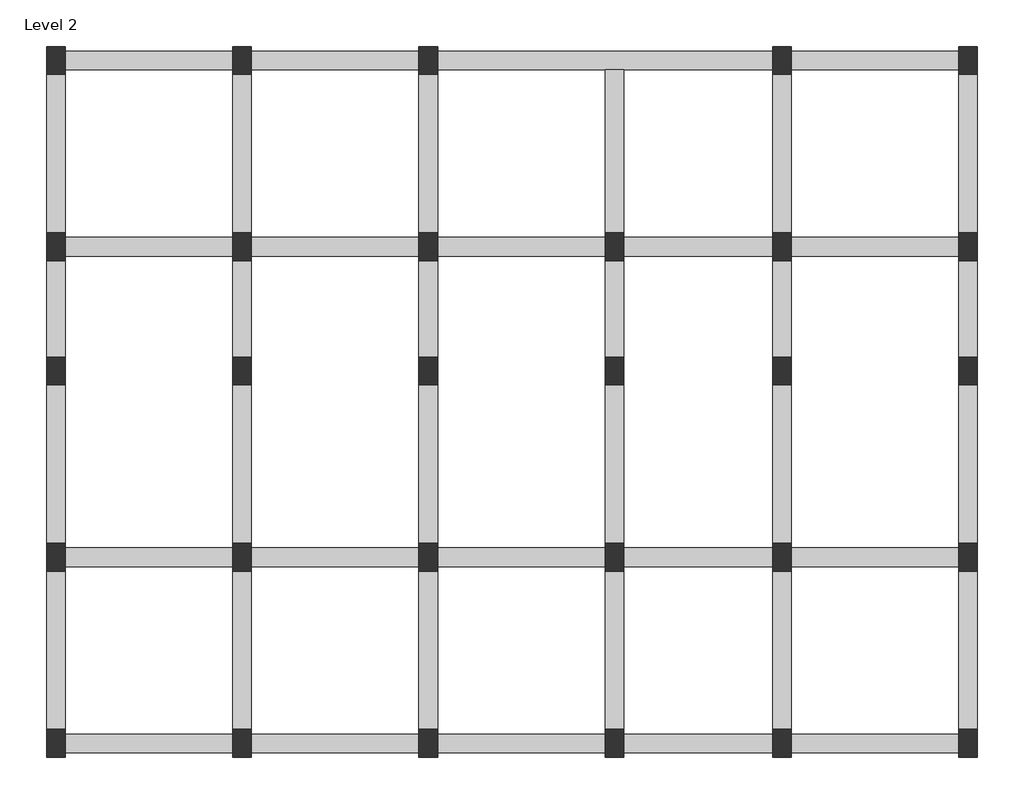
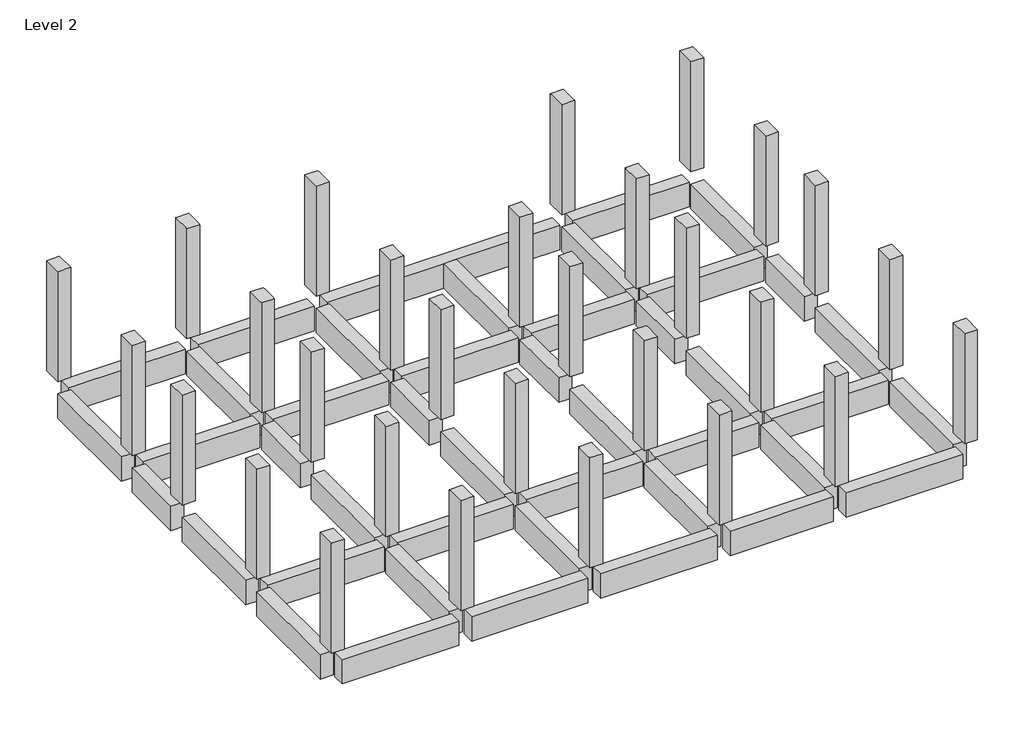
# One storey: 29 columns, 10 beams.
"""IFC4 building model written with IfcOpenShell, lengths in millimetres."""

from ifc_helpers import new_model, si_unit, frame, origin, place, context, project, spatial, polyline, outline, extrude, faceted_brep, element, save

model = new_model("IFC4")

# Units and contexts
model_context = context("Model", 3, world=origin())
ifc_project = project(units=[si_unit("LENGTHUNIT", "METRE", prefix="MILLI")], contexts=[model_context])

# Site, building, storey
site = spatial("IfcSite", under=ifc_project)
building = spatial("IfcBuilding", under=site)
storey = spatial("IfcBuildingStorey", under=building, Name="Level 2", Elevation=3048.0)

# Beams
placement = place(None, origin())
element("IfcBeam", 1, ObjectType="Concrete-Rectangular Beam : 12 x 24", at=placement, inside=storey, context=model_context, shape_type="SweptSolid", body=[
    extrude(outline(polyline([(2607.7603583, 7596.6647757), (2607.7603583, 7291.8647757), (-135.4396417, 7291.8647757), (-135.4396417, 7596.6647757), (2607.7603583, 7596.6647757)])), frame((0.0, 0.0, 2133.6), z_axis=(0.0, 0.0, 1.0), x_axis=(1.0, 0.0, 0.0)), (0.0, 0.0, 1.0), 609.6),
    extrude(outline(polyline([(-12022.6396417, 7291.8647757), (-12022.6396417, 7596.6647757), (-9279.4396417, 7596.6647757), (-9279.4396417, 7291.8647757), (-12022.6396417, 7291.8647757)])), frame((0.0, 0.0, 2133.6), z_axis=(0.0, 0.0, 1.0), x_axis=(1.0, 0.0, 0.0)), (0.0, 0.0, 1.0), 609.6),
    extrude(outline(polyline([(-8974.6396417, 7291.8647757), (-8974.6396417, 7596.6647757), (-6231.4396417, 7596.6647757), (-6231.4396417, 7291.8647757), (-8974.6396417, 7291.8647757)])), frame((0.0, 0.0, 2133.6), z_axis=(0.0, 0.0, 1.0), x_axis=(1.0, 0.0, 0.0)), (0.0, 0.0, 1.0), 609.6),
    extrude(outline(polyline([(-5926.6396417, 7291.8647757), (-5926.6396417, 7596.6647757), (-3183.4396417, 7596.6647757), (-3183.4396417, 7291.8647757), (-5926.6396417, 7291.8647757)])), frame((0.0, 0.0, 2133.6), z_axis=(0.0, 0.0, 1.0), x_axis=(1.0, 0.0, 0.0)), (0.0, 0.0, 1.0), 609.6),
    extrude(outline(polyline([(-2878.6396417, 7291.8647757), (-2878.6396417, 7596.6647757), (-440.2396417, 7596.6647757), (-440.2396417, 7291.8647757), (-2878.6396417, 7291.8647757)])), frame((0.0, 0.0, 2133.6), z_axis=(0.0, 0.0, 1.0), x_axis=(1.0, 0.0, 0.0)), (0.0, 0.0, 1.0), 609.6),
])
element("IfcBeam", 2, ObjectType="Concrete-Rectangular Beam : 12 x 24", at=placement, inside=storey, context=model_context, shape_type="SweptSolid", body=[
    extrude(outline(polyline([(2607.7603583, 10644.6647757), (2607.7603583, 10339.8647757), (-135.4396417, 10339.8647757), (-135.4396417, 10644.6647757), (2607.7603583, 10644.6647757)])), frame((0.0, 0.0, 2133.6), z_axis=(0.0, 0.0, 1.0), x_axis=(1.0, 0.0, 0.0)), (0.0, 0.0, 1.0), 609.6),
    extrude(outline(polyline([(-12022.6396417, 10339.8647757), (-12022.6396417, 10644.6647757), (-9279.4396417, 10644.6647757), (-9279.4396417, 10339.8647757), (-12022.6396417, 10339.8647757)])), frame((0.0, 0.0, 2133.6), z_axis=(0.0, 0.0, 1.0), x_axis=(1.0, 0.0, 0.0)), (0.0, 0.0, 1.0), 609.6),
    extrude(outline(polyline([(-8974.6396417, 10339.8647757), (-8974.6396417, 10644.6647757), (-6231.4396417, 10644.6647757), (-6231.4396417, 10339.8647757), (-8974.6396417, 10339.8647757)])), frame((0.0, 0.0, 2133.6), z_axis=(0.0, 0.0, 1.0), x_axis=(1.0, 0.0, 0.0)), (0.0, 0.0, 1.0), 609.6),
    extrude(outline(polyline([(-5926.6396417, 10339.8647757), (-5926.6396417, 10644.6647757), (-3183.4396417, 10644.6647757), (-3183.4396417, 10339.8647757), (-5926.6396417, 10339.8647757)])), frame((0.0, 0.0, 2133.6), z_axis=(0.0, 0.0, 1.0), x_axis=(1.0, 0.0, 0.0)), (0.0, 0.0, 1.0), 609.6),
    extrude(outline(polyline([(-2878.6396417, 10339.8647757), (-2878.6396417, 10644.6647757), (-440.2396417, 10644.6647757), (-440.2396417, 10339.8647757), (-2878.6396417, 10339.8647757)])), frame((0.0, 0.0, 2133.6), z_axis=(0.0, 0.0, 1.0), x_axis=(1.0, 0.0, 0.0)), (0.0, 0.0, 1.0), 609.6),
])
element("IfcBeam", 3, ObjectType="Concrete-Rectangular Beam : 12 x 24", at=placement, inside=storey, context=model_context, shape_type="SweptSolid", body=[
    extrude(outline(polyline([(2607.7603583, 15727.9119241), (2607.7603583, 15423.1119241), (-135.4396417, 15423.1119241), (-135.4396417, 15727.9119241), (2607.7603583, 15727.9119241)])), frame((0.0, 0.0, 2133.6), z_axis=(0.0, 0.0, 1.0), x_axis=(1.0, 0.0, 0.0)), (0.0, 0.0, 1.0), 609.6),
    extrude(outline(polyline([(-12022.6396417, 15423.1119241), (-12022.6396417, 15727.9119241), (-9279.4396417, 15727.9119241), (-9279.4396417, 15423.1119241), (-12022.6396417, 15423.1119241)])), frame((0.0, 0.0, 2133.6), z_axis=(0.0, 0.0, 1.0), x_axis=(1.0, 0.0, 0.0)), (0.0, 0.0, 1.0), 609.6),
    extrude(outline(polyline([(-8974.6396417, 15423.1119241), (-8974.6396417, 15727.9119241), (-6231.4396417, 15727.9119241), (-6231.4396417, 15423.1119241), (-8974.6396417, 15423.1119241)])), frame((0.0, 0.0, 2133.6), z_axis=(0.0, 0.0, 1.0), x_axis=(1.0, 0.0, 0.0)), (0.0, 0.0, 1.0), 609.6),
    extrude(outline(polyline([(-5926.6396417, 15423.1119241), (-5926.6396417, 15727.9119241), (-3183.4396417, 15727.9119241), (-3183.4396417, 15423.1119241), (-5926.6396417, 15423.1119241)])), frame((0.0, 0.0, 2133.6), z_axis=(0.0, 0.0, 1.0), x_axis=(1.0, 0.0, 0.0)), (0.0, 0.0, 1.0), 609.6),
    extrude(outline(polyline([(-2878.6396417, 15423.1119241), (-2878.6396417, 15727.9119241), (-440.2396417, 15727.9119241), (-440.2396417, 15423.1119241), (-2878.6396417, 15423.1119241)])), frame((0.0, 0.0, 2133.6), z_axis=(0.0, 0.0, 1.0), x_axis=(1.0, 0.0, 0.0)), (0.0, 0.0, 1.0), 609.6),
])
element("IfcBeam", 4, ObjectType="Concrete-Rectangular Beam : 12 x 24", at=placement, inside=storey, context=model_context, shape_type="Brep", body=[
    faceted_brep([(2607.7603583, 18471.1119241, 2743.2), (2607.7603583, 18775.9119241, 2743.2), (-135.4396417, 18775.9119241, 2743.2), (-135.4396417, 18471.1119241, 2743.2), (2607.7603583, 18471.1119241, 2133.6), (-135.4396417, 18471.1119241, 2133.6), (2607.7603583, 18775.9119241, 2133.6), (-135.4396417, 18775.9119241, 2133.6)], [[[0, 1, 2, 3]], [[4, 0, 3, 5]], [[6, 4, 5, 7]], [[1, 6, 7, 2]], [[1, 0, 4, 6]], [[3, 2, 7, 5]]]),
    faceted_brep([(-12022.6396417, 18471.1119241, 2743.2), (-12022.6396417, 18775.9119241, 2743.2), (-12022.6396417, 18775.9119241, 2133.6), (-12022.6396417, 18471.1119241, 2133.6), (-9279.4396417, 18775.9119241, 2743.2), (-9279.4396417, 18471.1119241, 2743.2), (-9279.4396417, 18471.1119241, 2133.6), (-9279.4396417, 18775.9119241, 2133.6)], [[[0, 1, 2, 3]], [[4, 5, 6, 7]], [[1, 0, 5, 4]], [[0, 3, 6, 5]], [[3, 2, 7, 6]], [[2, 1, 4, 7]]]),
    faceted_brep([(-8974.6396417, 18471.1119241, 2743.2), (-8974.6396417, 18775.9119241, 2743.2), (-8974.6396417, 18775.9119241, 2133.6), (-8974.6396417, 18471.1119241, 2133.6), (-6231.4396417, 18775.9119241, 2743.2), (-6231.4396417, 18471.1119241, 2743.2), (-6231.4396417, 18471.1119241, 2133.6), (-6231.4396417, 18775.9119241, 2133.6)], [[[0, 1, 2, 3]], [[4, 5, 6, 7]], [[1, 0, 5, 4]], [[0, 3, 6, 5]], [[3, 2, 7, 6]], [[2, 1, 4, 7]]]),
    faceted_brep([(-5926.6396417, 18471.1119241, 2743.2), (-5926.6396417, 18775.9119241, 2743.2), (-5926.6396417, 18775.9119241, 2133.6), (-5926.6396417, 18471.1119241, 2133.6), (-440.2396417, 18775.9119241, 2743.2), (-440.2396417, 18471.1119241, 2743.2), (-440.2396417, 18471.1119241, 2133.6), (-440.2396417, 18775.9119241, 2133.6), (-3183.4396417, 18471.1119241, 2743.2), (-2878.6396417, 18471.1119241, 2743.2), (-3183.4396417, 18471.1119241, 2133.6), (-2878.6396417, 18471.1119241, 2133.6)], [[[0, 1, 2, 3]], [[4, 5, 6, 7]], [[1, 0, 8, 9, 5, 4]], [[0, 3, 10, 11, 6, 5, 9, 8]], [[3, 2, 7, 6, 11, 10]], [[2, 1, 4, 7]]]),
])
element("IfcBeam", 5, ObjectType="Concrete-Rectangular Beam : 12 x 24", at=placement, inside=storey, context=model_context, shape_type="SweptSolid", body=[
    extrude(outline(polyline([(-12022.6396417, 7672.8647757), (-12327.4396417, 7672.8647757), (-12327.4396417, 10263.6647757), (-12022.6396417, 10263.6647757), (-12022.6396417, 7672.8647757)])), frame((0.0, 0.0, 2133.6), z_axis=(0.0, 0.0, 1.0), x_axis=(1.0, 0.0, 0.0)), (0.0, 0.0, 1.0), 609.6),
    extrude(outline(polyline([(-12327.4396417, 18394.9119241), (-12022.6396417, 18394.9119241), (-12022.6396417, 15804.1119241), (-12327.4396417, 15804.1119241), (-12327.4396417, 18394.9119241)])), frame((0.0, 0.0, 2133.6), z_axis=(0.0, 0.0, 1.0), x_axis=(1.0, 0.0, 0.0)), (0.0, 0.0, 1.0), 609.6),
    extrude(outline(polyline([(-12022.6396417, 10720.8647757), (-12327.4396417, 10720.8647757), (-12327.4396417, 13311.6647757), (-12022.6396417, 13311.6647757), (-12022.6396417, 10720.8647757)])), frame((0.0, 0.0, 2133.6), z_axis=(0.0, 0.0, 1.0), x_axis=(1.0, 0.0, 0.0)), (0.0, 0.0, 1.0), 609.6),
    extrude(outline(polyline([(-12022.6396417, 13768.8647757), (-12327.4396417, 13768.8647757), (-12327.4396417, 15346.9119241), (-12022.6396417, 15346.9119241), (-12022.6396417, 13768.8647757)])), frame((0.0, 0.0, 2133.6), z_axis=(0.0, 0.0, 1.0), x_axis=(1.0, 0.0, 0.0)), (0.0, 0.0, 1.0), 609.6),
])
element("IfcBeam", 6, ObjectType="Concrete-Rectangular Beam : 12 x 24", at=placement, inside=storey, context=model_context, shape_type="SweptSolid", body=[
    extrude(outline(polyline([(-8974.6396417, 7672.8647757), (-9279.4396417, 7672.8647757), (-9279.4396417, 10263.6647757), (-8974.6396417, 10263.6647757), (-8974.6396417, 7672.8647757)])), frame((0.0, 0.0, 2133.6), z_axis=(0.0, 0.0, 1.0), x_axis=(1.0, 0.0, 0.0)), (0.0, 0.0, 1.0), 609.6),
    extrude(outline(polyline([(-9279.4396417, 18394.9119241), (-8974.6396417, 18394.9119241), (-8974.6396417, 15804.1119241), (-9279.4396417, 15804.1119241), (-9279.4396417, 18394.9119241)])), frame((0.0, 0.0, 2133.6), z_axis=(0.0, 0.0, 1.0), x_axis=(1.0, 0.0, 0.0)), (0.0, 0.0, 1.0), 609.6),
    extrude(outline(polyline([(-8974.6396417, 10720.8647757), (-9279.4396417, 10720.8647757), (-9279.4396417, 13311.6647757), (-8974.6396417, 13311.6647757), (-8974.6396417, 10720.8647757)])), frame((0.0, 0.0, 2133.6), z_axis=(0.0, 0.0, 1.0), x_axis=(1.0, 0.0, 0.0)), (0.0, 0.0, 1.0), 609.6),
    extrude(outline(polyline([(-8974.6396417, 13768.8647757), (-9279.4396417, 13768.8647757), (-9279.4396417, 15346.9119241), (-8974.6396417, 15346.9119241), (-8974.6396417, 13768.8647757)])), frame((0.0, 0.0, 2133.6), z_axis=(0.0, 0.0, 1.0), x_axis=(1.0, 0.0, 0.0)), (0.0, 0.0, 1.0), 609.6),
])
element("IfcBeam", 7, ObjectType="Concrete-Rectangular Beam : 12 x 24", at=placement, inside=storey, context=model_context, shape_type="SweptSolid", body=[
    extrude(outline(polyline([(-5926.6396417, 7672.8647757), (-6231.4396417, 7672.8647757), (-6231.4396417, 10263.6647757), (-5926.6396417, 10263.6647757), (-5926.6396417, 7672.8647757)])), frame((0.0, 0.0, 2133.6), z_axis=(0.0, 0.0, 1.0), x_axis=(1.0, 0.0, 0.0)), (0.0, 0.0, 1.0), 609.6),
    extrude(outline(polyline([(-6231.4396417, 18394.9119241), (-5926.6396417, 18394.9119241), (-5926.6396417, 15804.1119241), (-6231.4396417, 15804.1119241), (-6231.4396417, 18394.9119241)])), frame((0.0, 0.0, 2133.6), z_axis=(0.0, 0.0, 1.0), x_axis=(1.0, 0.0, 0.0)), (0.0, 0.0, 1.0), 609.6),
    extrude(outline(polyline([(-5926.6396417, 10720.8647757), (-6231.4396417, 10720.8647757), (-6231.4396417, 13311.6647757), (-5926.6396417, 13311.6647757), (-5926.6396417, 10720.8647757)])), frame((0.0, 0.0, 2133.6), z_axis=(0.0, 0.0, 1.0), x_axis=(1.0, 0.0, 0.0)), (0.0, 0.0, 1.0), 609.6),
    extrude(outline(polyline([(-5926.6396417, 13768.8647757), (-6231.4396417, 13768.8647757), (-6231.4396417, 15346.9119241), (-5926.6396417, 15346.9119241), (-5926.6396417, 13768.8647757)])), frame((0.0, 0.0, 2133.6), z_axis=(0.0, 0.0, 1.0), x_axis=(1.0, 0.0, 0.0)), (0.0, 0.0, 1.0), 609.6),
])
element("IfcBeam", 8, ObjectType="Concrete-Rectangular Beam : 12 x 24", at=placement, inside=storey, context=model_context, shape_type="SweptSolid", body=[
    extrude(outline(polyline([(-2878.6396417, 7672.8647757), (-3183.4396417, 7672.8647757), (-3183.4396417, 10263.6647757), (-2878.6396417, 10263.6647757), (-2878.6396417, 7672.8647757)])), frame((0.0, 0.0, 2133.6), z_axis=(0.0, 0.0, 1.0), x_axis=(1.0, 0.0, 0.0)), (0.0, 0.0, 1.0), 609.6),
    extrude(outline(polyline([(-2878.6396417, 10720.8647757), (-3183.4396417, 10720.8647757), (-3183.4396417, 13311.6647757), (-2878.6396417, 13311.6647757), (-2878.6396417, 10720.8647757)])), frame((0.0, 0.0, 2133.6), z_axis=(0.0, 0.0, 1.0), x_axis=(1.0, 0.0, 0.0)), (0.0, 0.0, 1.0), 609.6),
    extrude(outline(polyline([(-2878.6396417, 13768.8647757), (-3183.4396417, 13768.8647757), (-3183.4396417, 15346.9119241), (-2878.6396417, 15346.9119241), (-2878.6396417, 13768.8647757)])), frame((0.0, 0.0, 2133.6), z_axis=(0.0, 0.0, 1.0), x_axis=(1.0, 0.0, 0.0)), (0.0, 0.0, 1.0), 609.6),
    extrude(outline(polyline([(-2878.6396417, 15804.1119241), (-3183.4396417, 15804.1119241), (-3183.4396417, 18471.1119241), (-2878.6396417, 18471.1119241), (-2878.6396417, 15804.1119241)])), frame((0.0, 0.0, 2133.6), z_axis=(0.0, 0.0, 1.0), x_axis=(1.0, 0.0, 0.0)), (0.0, 0.0, 1.0), 609.6),
])
element("IfcBeam", 9, ObjectType="Concrete-Rectangular Beam : 12 x 24", at=placement, inside=storey, context=model_context, shape_type="SweptSolid", body=[
    extrude(outline(polyline([(-135.4396417, 7672.8647757), (-440.2396417, 7672.8647757), (-440.2396417, 10263.6647757), (-135.4396417, 10263.6647757), (-135.4396417, 7672.8647757)])), frame((0.0, 0.0, 2133.6), z_axis=(0.0, 0.0, 1.0), x_axis=(1.0, 0.0, 0.0)), (0.0, 0.0, 1.0), 609.6),
    extrude(outline(polyline([(-440.2396417, 18394.9119241), (-135.4396417, 18394.9119241), (-135.4396417, 15804.1119241), (-440.2396417, 15804.1119241), (-440.2396417, 18394.9119241)])), frame((0.0, 0.0, 2133.6), z_axis=(0.0, 0.0, 1.0), x_axis=(1.0, 0.0, 0.0)), (0.0, 0.0, 1.0), 609.6),
    extrude(outline(polyline([(-135.4396417, 10720.8647757), (-440.2396417, 10720.8647757), (-440.2396417, 13311.6647757), (-135.4396417, 13311.6647757), (-135.4396417, 10720.8647757)])), frame((0.0, 0.0, 2133.6), z_axis=(0.0, 0.0, 1.0), x_axis=(1.0, 0.0, 0.0)), (0.0, 0.0, 1.0), 609.6),
    extrude(outline(polyline([(-135.4396417, 13768.8647757), (-440.2396417, 13768.8647757), (-440.2396417, 15346.9119241), (-135.4396417, 15346.9119241), (-135.4396417, 13768.8647757)])), frame((0.0, 0.0, 2133.6), z_axis=(0.0, 0.0, 1.0), x_axis=(1.0, 0.0, 0.0)), (0.0, 0.0, 1.0), 609.6),
])
element("IfcBeam", 10, ObjectType="Concrete-Rectangular Beam : 12 x 24", at=placement, inside=storey, context=model_context, shape_type="SweptSolid", body=[
    extrude(outline(polyline([(2912.5603583, 7672.8647757), (2607.7603583, 7672.8647757), (2607.7603583, 10263.6647757), (2912.5603583, 10263.6647757), (2912.5603583, 7672.8647757)])), frame((0.0, 0.0, 2133.6), z_axis=(0.0, 0.0, 1.0), x_axis=(1.0, 0.0, 0.0)), (0.0, 0.0, 1.0), 609.6),
    extrude(outline(polyline([(2607.7603583, 18394.9119241), (2912.5603583, 18394.9119241), (2912.5603583, 15804.1119241), (2607.7603583, 15804.1119241), (2607.7603583, 18394.9119241)])), frame((0.0, 0.0, 2133.6), z_axis=(0.0, 0.0, 1.0), x_axis=(1.0, 0.0, 0.0)), (0.0, 0.0, 1.0), 609.6),
    extrude(outline(polyline([(2912.5603583, 10720.8647757), (2607.7603583, 10720.8647757), (2607.7603583, 13311.6647757), (2912.5603583, 13311.6647757), (2912.5603583, 10720.8647757)])), frame((0.0, 0.0, 2133.6), z_axis=(0.0, 0.0, 1.0), x_axis=(1.0, 0.0, 0.0)), (0.0, 0.0, 1.0), 609.6),
    extrude(outline(polyline([(2912.5603583, 13768.8647757), (2607.7603583, 13768.8647757), (2607.7603583, 15346.9119241), (2912.5603583, 15346.9119241), (2912.5603583, 13768.8647757)])), frame((0.0, 0.0, 2133.6), z_axis=(0.0, 0.0, 1.0), x_axis=(1.0, 0.0, 0.0)), (0.0, 0.0, 1.0), 609.6),
])

# Columns
element("IfcColumn", 11, ObjectType="Concrete-Rectangular-Column : c1", at=placement, inside=storey, context=model_context, shape_type="SweptSolid", body=[
    extrude(outline(polyline([(-12327.4396417, 7215.6647757), (-12327.4396417, 7672.8647757), (-12022.6396417, 7672.8647757), (-12022.6396417, 7215.6647757), (-12327.4396417, 7215.6647757)])), frame((0.0, 0.0, 3048.0), z_axis=(0.0, 0.0, 1.0), x_axis=(1.0, 0.0, 0.0)), (0.0, 0.0, 1.0), 2743.2),
])
element("IfcColumn", 12, ObjectType="Concrete-Rectangular-Column : c1", at=placement, inside=storey, context=model_context, shape_type="Brep", body=[
    faceted_brep([(-9279.4396417, 7215.6647757, 3048.0), (-9279.4396417, 7672.8647757, 3048.0), (-8974.6396417, 7672.8647757, 3048.0), (-8974.6396417, 7215.6647757, 3048.0), (-9279.4396417, 7215.6647757, 5791.2), (-9279.4396417, 7291.8647757, 5791.2), (-9279.4396417, 7596.6647757, 5791.2), (-9279.4396417, 7672.8647757, 5791.2), (-8974.6396417, 7672.8647757, 5791.2), (-8974.6396417, 7596.6647757, 5791.2), (-8974.6396417, 7291.8647757, 5791.2), (-8974.6396417, 7215.6647757, 5791.2)], [[[0, 1, 2, 3]], [[4, 5, 6, 7, 1, 0]], [[7, 8, 2, 1]], [[8, 9, 10, 11, 3, 2]], [[11, 4, 0, 3]], [[4, 11, 10, 9, 8, 7, 6, 5]]]),
])
element("IfcColumn", 13, ObjectType="Concrete-Rectangular-Column : c1", at=placement, inside=storey, context=model_context, shape_type="Brep", body=[
    faceted_brep([(-6231.4396417, 7215.6647757, 3048.0), (-6231.4396417, 7672.8647757, 3048.0), (-5926.6396417, 7672.8647757, 3048.0), (-5926.6396417, 7215.6647757, 3048.0), (-6231.4396417, 7215.6647757, 5791.2), (-6231.4396417, 7291.8647757, 5791.2), (-6231.4396417, 7596.6647757, 5791.2), (-6231.4396417, 7672.8647757, 5791.2), (-5926.6396417, 7672.8647757, 5791.2), (-5926.6396417, 7596.6647757, 5791.2), (-5926.6396417, 7291.8647757, 5791.2), (-5926.6396417, 7215.6647757, 5791.2)], [[[0, 1, 2, 3]], [[4, 5, 6, 7, 1, 0]], [[7, 8, 2, 1]], [[8, 9, 10, 11, 3, 2]], [[11, 4, 0, 3]], [[4, 11, 10, 9, 8, 7, 6, 5]]]),
])
element("IfcColumn", 14, ObjectType="Concrete-Rectangular-Column : c1", at=placement, inside=storey, context=model_context, shape_type="Brep", body=[
    faceted_brep([(-3183.4396417, 7215.6647757, 3048.0), (-3183.4396417, 7672.8647757, 3048.0), (-2878.6396417, 7672.8647757, 3048.0), (-2878.6396417, 7215.6647757, 3048.0), (-3183.4396417, 7215.6647757, 5791.2), (-3183.4396417, 7291.8647757, 5791.2), (-3183.4396417, 7596.6647757, 5791.2), (-3183.4396417, 7672.8647757, 5791.2), (-2878.6396417, 7672.8647757, 5791.2), (-2878.6396417, 7596.6647757, 5791.2), (-2878.6396417, 7291.8647757, 5791.2), (-2878.6396417, 7215.6647757, 5791.2)], [[[0, 1, 2, 3]], [[4, 5, 6, 7, 1, 0]], [[7, 8, 2, 1]], [[8, 9, 10, 11, 3, 2]], [[11, 4, 0, 3]], [[4, 11, 10, 9, 8, 7, 6, 5]]]),
])
element("IfcColumn", 15, ObjectType="Concrete-Rectangular-Column : c1", at=placement, inside=storey, context=model_context, shape_type="Brep", body=[
    faceted_brep([(-440.2396417, 7215.6647757, 3048.0), (-440.2396417, 7672.8647757, 3048.0), (-135.4396417, 7672.8647757, 3048.0), (-135.4396417, 7215.6647757, 3048.0), (-440.2396417, 7215.6647757, 5791.2), (-440.2396417, 7291.8647757, 5791.2), (-440.2396417, 7596.6647757, 5791.2), (-440.2396417, 7672.8647757, 5791.2), (-135.4396417, 7672.8647757, 5791.2), (-135.4396417, 7596.6647757, 5791.2), (-135.4396417, 7291.8647757, 5791.2), (-135.4396417, 7215.6647757, 5791.2)], [[[0, 1, 2, 3]], [[4, 5, 6, 7, 1, 0]], [[7, 8, 2, 1]], [[8, 9, 10, 11, 3, 2]], [[11, 4, 0, 3]], [[4, 11, 10, 9, 8, 7, 6, 5]]]),
])
element("IfcColumn", 16, ObjectType="Concrete-Rectangular-Column : c1", at=placement, inside=storey, context=model_context, shape_type="SweptSolid", body=[
    extrude(outline(polyline([(2607.7603583, 7215.6647757), (2607.7603583, 7672.8647757), (2912.5603583, 7672.8647757), (2912.5603583, 7215.6647757), (2607.7603583, 7215.6647757)])), frame((0.0, 0.0, 3048.0), z_axis=(0.0, 0.0, 1.0), x_axis=(1.0, 0.0, 0.0)), (0.0, 0.0, 1.0), 2743.2),
])
element("IfcColumn", 17, ObjectType="Concrete-Rectangular-Column : c1", at=placement, inside=storey, context=model_context, shape_type="Brep", body=[
    faceted_brep([(-12327.4396417, 10263.6647757, 3048.0), (-12327.4396417, 10720.8647757, 3048.0), (-12022.6396417, 10720.8647757, 3048.0), (-12022.6396417, 10263.6647757, 3048.0), (-12327.4396417, 10263.6647757, 5791.2), (-12327.4396417, 10720.8647757, 5791.2), (-12327.4396417, 10720.8647757, 5181.6), (-12327.4396417, 10263.6647757, 5181.6), (-12022.6396417, 10720.8647757, 5791.2), (-12022.6396417, 10720.8647757, 5181.6), (-12022.6396417, 10263.6647757, 5791.2), (-12022.6396417, 10263.6647757, 5181.6)], [[[0, 1, 2, 3]], [[4, 5, 6, 1, 0, 7]], [[5, 8, 9, 2, 1, 6]], [[8, 10, 11, 3, 2, 9]], [[10, 4, 7, 0, 3, 11]], [[4, 10, 8, 5]]]),
])
element("IfcColumn", 18, ObjectType="Concrete-Rectangular-Column : c1", at=placement, inside=storey, context=model_context, shape_type="Brep", body=[
    faceted_brep([(-9279.4396417, 10263.6647757, 3048.0), (-9279.4396417, 10720.8647757, 3048.0), (-8974.6396417, 10720.8647757, 3048.0), (-8974.6396417, 10263.6647757, 3048.0), (-9279.4396417, 10263.6647757, 5791.2), (-9279.4396417, 10339.8647757, 5791.2), (-9279.4396417, 10644.6647757, 5791.2), (-9279.4396417, 10720.8647757, 5791.2), (-9279.4396417, 10720.8647757, 5181.6), (-9279.4396417, 10263.6647757, 5181.6), (-8974.6396417, 10720.8647757, 5791.2), (-8974.6396417, 10720.8647757, 5181.6), (-8974.6396417, 10644.6647757, 5791.2), (-8974.6396417, 10339.8647757, 5791.2), (-8974.6396417, 10263.6647757, 5791.2), (-8974.6396417, 10263.6647757, 5181.6)], [[[0, 1, 2, 3]], [[4, 5, 6, 7, 8, 1, 0, 9]], [[7, 10, 11, 2, 1, 8]], [[10, 12, 13, 14, 15, 3, 2, 11]], [[14, 4, 9, 0, 3, 15]], [[4, 14, 13, 12, 10, 7, 6, 5]]]),
])
element("IfcColumn", 19, ObjectType="Concrete-Rectangular-Column : c1", at=placement, inside=storey, context=model_context, shape_type="Brep", body=[
    faceted_brep([(-6231.4396417, 10263.6647757, 3048.0), (-6231.4396417, 10720.8647757, 3048.0), (-5926.6396417, 10720.8647757, 3048.0), (-5926.6396417, 10263.6647757, 3048.0), (-6231.4396417, 10263.6647757, 5791.2), (-6231.4396417, 10339.8647757, 5791.2), (-6231.4396417, 10644.6647757, 5791.2), (-6231.4396417, 10720.8647757, 5791.2), (-6231.4396417, 10720.8647757, 5181.6), (-6231.4396417, 10263.6647757, 5181.6), (-5926.6396417, 10720.8647757, 5791.2), (-5926.6396417, 10720.8647757, 5181.6), (-5926.6396417, 10644.6647757, 5791.2), (-5926.6396417, 10339.8647757, 5791.2), (-5926.6396417, 10263.6647757, 5791.2), (-5926.6396417, 10263.6647757, 5181.6)], [[[0, 1, 2, 3]], [[4, 5, 6, 7, 8, 1, 0, 9]], [[7, 10, 11, 2, 1, 8]], [[10, 12, 13, 14, 15, 3, 2, 11]], [[14, 4, 9, 0, 3, 15]], [[4, 14, 13, 12, 10, 7, 6, 5]]]),
])
element("IfcColumn", 20, ObjectType="Concrete-Rectangular-Column : c1", at=placement, inside=storey, context=model_context, shape_type="Brep", body=[
    faceted_brep([(-3183.4396417, 10263.6647757, 3048.0), (-3183.4396417, 10720.8647757, 3048.0), (-2878.6396417, 10720.8647757, 3048.0), (-2878.6396417, 10263.6647757, 3048.0), (-3183.4396417, 10263.6647757, 5791.2), (-3183.4396417, 10339.8647757, 5791.2), (-3183.4396417, 10644.6647757, 5791.2), (-3183.4396417, 10720.8647757, 5791.2), (-2878.6396417, 10720.8647757, 5791.2), (-2878.6396417, 10644.6647757, 5791.2), (-2878.6396417, 10339.8647757, 5791.2), (-2878.6396417, 10263.6647757, 5791.2)], [[[0, 1, 2, 3]], [[4, 5, 6, 7, 1, 0]], [[7, 8, 2, 1]], [[8, 9, 10, 11, 3, 2]], [[11, 4, 0, 3]], [[4, 11, 10, 9, 8, 7, 6, 5]]]),
])
element("IfcColumn", 21, ObjectType="Concrete-Rectangular-Column : c1", at=placement, inside=storey, context=model_context, shape_type="Brep", body=[
    faceted_brep([(-440.2396417, 10263.6647757, 3048.0), (-440.2396417, 10720.8647757, 3048.0), (-135.4396417, 10720.8647757, 3048.0), (-135.4396417, 10263.6647757, 3048.0), (-440.2396417, 10263.6647757, 5791.2), (-440.2396417, 10339.8647757, 5791.2), (-440.2396417, 10644.6647757, 5791.2), (-440.2396417, 10720.8647757, 5791.2), (-440.2396417, 10720.8647757, 5181.6), (-440.2396417, 10263.6647757, 5181.6), (-135.4396417, 10720.8647757, 5791.2), (-135.4396417, 10720.8647757, 5181.6), (-135.4396417, 10644.6647757, 5791.2), (-135.4396417, 10339.8647757, 5791.2), (-135.4396417, 10263.6647757, 5791.2), (-135.4396417, 10263.6647757, 5181.6)], [[[0, 1, 2, 3]], [[4, 5, 6, 7, 8, 1, 0, 9]], [[7, 10, 11, 2, 1, 8]], [[10, 12, 13, 14, 15, 3, 2, 11]], [[14, 4, 9, 0, 3, 15]], [[4, 14, 13, 12, 10, 7, 6, 5]]]),
])
element("IfcColumn", 22, ObjectType="Concrete-Rectangular-Column : c1", at=placement, inside=storey, context=model_context, shape_type="Brep", body=[
    faceted_brep([(2607.7603583, 10263.6647757, 3048.0), (2607.7603583, 10720.8647757, 3048.0), (2912.5603583, 10720.8647757, 3048.0), (2912.5603583, 10263.6647757, 3048.0), (2607.7603583, 10263.6647757, 5791.2), (2607.7603583, 10720.8647757, 5791.2), (2607.7603583, 10720.8647757, 5181.6), (2607.7603583, 10263.6647757, 5181.6), (2912.5603583, 10720.8647757, 5791.2), (2912.5603583, 10720.8647757, 5181.6), (2912.5603583, 10263.6647757, 5791.2), (2912.5603583, 10263.6647757, 5181.6)], [[[0, 1, 2, 3]], [[4, 5, 6, 1, 0, 7]], [[5, 8, 9, 2, 1, 6]], [[8, 10, 11, 3, 2, 9]], [[10, 4, 7, 0, 3, 11]], [[4, 10, 8, 5]]]),
])
element("IfcColumn", 23, ObjectType="Concrete-Rectangular-Column : c1", at=placement, inside=storey, context=model_context, shape_type="Brep", body=[
    faceted_brep([(-12327.4396417, 13311.6647757, 3048.0), (-12327.4396417, 13768.8647757, 3048.0), (-12022.6396417, 13768.8647757, 3048.0), (-12022.6396417, 13311.6647757, 3048.0), (-12327.4396417, 13311.6647757, 5791.2), (-12327.4396417, 13768.8647757, 5791.2), (-12327.4396417, 13768.8647757, 5181.6), (-12327.4396417, 13311.6647757, 5181.6), (-12022.6396417, 13768.8647757, 5791.2), (-12022.6396417, 13768.8647757, 5181.6), (-12022.6396417, 13311.6647757, 5791.2), (-12022.6396417, 13311.6647757, 5181.6)], [[[0, 1, 2, 3]], [[4, 5, 6, 1, 0, 7]], [[5, 8, 9, 2, 1, 6]], [[8, 10, 11, 3, 2, 9]], [[10, 4, 7, 0, 3, 11]], [[4, 10, 8, 5]]]),
])
element("IfcColumn", 24, ObjectType="Concrete-Rectangular-Column : c1", at=placement, inside=storey, context=model_context, shape_type="Brep", body=[
    faceted_brep([(-9279.4396417, 13311.6647757, 3048.0), (-9279.4396417, 13768.8647757, 3048.0), (-8974.6396417, 13768.8647757, 3048.0), (-8974.6396417, 13311.6647757, 3048.0), (-9279.4396417, 13311.6647757, 5791.2), (-9279.4396417, 13768.8647757, 5791.2), (-9279.4396417, 13768.8647757, 5181.6), (-9279.4396417, 13311.6647757, 5181.6), (-8974.6396417, 13768.8647757, 5791.2), (-8974.6396417, 13768.8647757, 5181.6), (-8974.6396417, 13311.6647757, 5791.2), (-8974.6396417, 13311.6647757, 5181.6)], [[[0, 1, 2, 3]], [[4, 5, 6, 1, 0, 7]], [[5, 8, 9, 2, 1, 6]], [[8, 10, 11, 3, 2, 9]], [[10, 4, 7, 0, 3, 11]], [[4, 10, 8, 5]]]),
])
element("IfcColumn", 25, ObjectType="Concrete-Rectangular-Column : c1", at=placement, inside=storey, context=model_context, shape_type="Brep", body=[
    faceted_brep([(-6231.4396417, 13311.6647757, 3048.0), (-6231.4396417, 13768.8647757, 3048.0), (-5926.6396417, 13768.8647757, 3048.0), (-5926.6396417, 13311.6647757, 3048.0), (-6231.4396417, 13311.6647757, 5791.2), (-6231.4396417, 13768.8647757, 5791.2), (-6231.4396417, 13768.8647757, 5181.6), (-6231.4396417, 13311.6647757, 5181.6), (-5926.6396417, 13768.8647757, 5791.2), (-5926.6396417, 13768.8647757, 5181.6), (-5926.6396417, 13311.6647757, 5791.2), (-5926.6396417, 13311.6647757, 5181.6)], [[[0, 1, 2, 3]], [[4, 5, 6, 1, 0, 7]], [[5, 8, 9, 2, 1, 6]], [[8, 10, 11, 3, 2, 9]], [[10, 4, 7, 0, 3, 11]], [[4, 10, 8, 5]]]),
])
element("IfcColumn", 26, ObjectType="Concrete-Rectangular-Column : c1", at=placement, inside=storey, context=model_context, shape_type="SweptSolid", body=[
    extrude(outline(polyline([(-3183.4396417, 13311.6647757), (-3183.4396417, 13768.8647757), (-2878.6396417, 13768.8647757), (-2878.6396417, 13311.6647757), (-3183.4396417, 13311.6647757)])), frame((0.0, 0.0, 3048.0), z_axis=(0.0, 0.0, 1.0), x_axis=(1.0, 0.0, 0.0)), (0.0, 0.0, 1.0), 2743.2),
])
element("IfcColumn", 27, ObjectType="Concrete-Rectangular-Column : c1", at=placement, inside=storey, context=model_context, shape_type="Brep", body=[
    faceted_brep([(-440.2396417, 13311.6647757, 3048.0), (-440.2396417, 13768.8647757, 3048.0), (-135.4396417, 13768.8647757, 3048.0), (-135.4396417, 13311.6647757, 3048.0), (-440.2396417, 13311.6647757, 5791.2), (-440.2396417, 13768.8647757, 5791.2), (-440.2396417, 13768.8647757, 5181.6), (-440.2396417, 13311.6647757, 5181.6), (-135.4396417, 13768.8647757, 5791.2), (-135.4396417, 13768.8647757, 5181.6), (-135.4396417, 13311.6647757, 5791.2), (-135.4396417, 13311.6647757, 5181.6)], [[[0, 1, 2, 3]], [[4, 5, 6, 1, 0, 7]], [[5, 8, 9, 2, 1, 6]], [[8, 10, 11, 3, 2, 9]], [[10, 4, 7, 0, 3, 11]], [[4, 10, 8, 5]]]),
])
element("IfcColumn", 28, ObjectType="Concrete-Rectangular-Column : c1", at=placement, inside=storey, context=model_context, shape_type="Brep", body=[
    faceted_brep([(2607.7603583, 13311.6647757, 3048.0), (2607.7603583, 13768.8647757, 3048.0), (2912.5603583, 13768.8647757, 3048.0), (2912.5603583, 13311.6647757, 3048.0), (2607.7603583, 13311.6647757, 5791.2), (2607.7603583, 13768.8647757, 5791.2), (2607.7603583, 13768.8647757, 5181.6), (2607.7603583, 13311.6647757, 5181.6), (2912.5603583, 13768.8647757, 5791.2), (2912.5603583, 13768.8647757, 5181.6), (2912.5603583, 13311.6647757, 5791.2), (2912.5603583, 13311.6647757, 5181.6)], [[[0, 1, 2, 3]], [[4, 5, 6, 1, 0, 7]], [[5, 8, 9, 2, 1, 6]], [[8, 10, 11, 3, 2, 9]], [[10, 4, 7, 0, 3, 11]], [[4, 10, 8, 5]]]),
])
element("IfcColumn", 29, ObjectType="Concrete-Rectangular-Column : c1", at=placement, inside=storey, context=model_context, shape_type="Brep", body=[
    faceted_brep([(-12327.4396417, 15346.9119241, 3048.0), (-12327.4396417, 15804.1119241, 3048.0), (-12022.6396417, 15804.1119241, 3048.0), (-12022.6396417, 15346.9119241, 3048.0), (-12327.4396417, 15346.9119241, 5791.2), (-12327.4396417, 15804.1119241, 5791.2), (-12327.4396417, 15804.1119241, 5181.6), (-12327.4396417, 15346.9119241, 5181.6), (-12022.6396417, 15804.1119241, 5791.2), (-12022.6396417, 15804.1119241, 5181.6), (-12022.6396417, 15346.9119241, 5791.2), (-12022.6396417, 15346.9119241, 5181.6)], [[[0, 1, 2, 3]], [[4, 5, 6, 1, 0, 7]], [[5, 8, 9, 2, 1, 6]], [[8, 10, 11, 3, 2, 9]], [[10, 4, 7, 0, 3, 11]], [[4, 10, 8, 5]]]),
])
element("IfcColumn", 30, ObjectType="Concrete-Rectangular-Column : c1", at=placement, inside=storey, context=model_context, shape_type="Brep", body=[
    faceted_brep([(-9279.4396417, 15346.9119241, 3048.0), (-9279.4396417, 15804.1119241, 3048.0), (-8974.6396417, 15804.1119241, 3048.0), (-8974.6396417, 15346.9119241, 3048.0), (-9279.4396417, 15346.9119241, 5791.2), (-9279.4396417, 15423.1119241, 5791.2), (-9279.4396417, 15727.9119241, 5791.2), (-9279.4396417, 15804.1119241, 5791.2), (-9279.4396417, 15804.1119241, 5181.6), (-9279.4396417, 15346.9119241, 5181.6), (-8974.6396417, 15804.1119241, 5791.2), (-8974.6396417, 15804.1119241, 5181.6), (-8974.6396417, 15727.9119241, 5791.2), (-8974.6396417, 15423.1119241, 5791.2), (-8974.6396417, 15346.9119241, 5791.2), (-8974.6396417, 15346.9119241, 5181.6)], [[[0, 1, 2, 3]], [[4, 5, 6, 7, 8, 1, 0, 9]], [[7, 10, 11, 2, 1, 8]], [[10, 12, 13, 14, 15, 3, 2, 11]], [[14, 4, 9, 0, 3, 15]], [[4, 14, 13, 12, 10, 7, 6, 5]]]),
])
element("IfcColumn", 31, ObjectType="Concrete-Rectangular-Column : c1", at=placement, inside=storey, context=model_context, shape_type="Brep", body=[
    faceted_brep([(-6231.4396417, 15346.9119241, 3048.0), (-6231.4396417, 15804.1119241, 3048.0), (-5926.6396417, 15804.1119241, 3048.0), (-5926.6396417, 15346.9119241, 3048.0), (-6231.4396417, 15346.9119241, 5791.2), (-6231.4396417, 15423.1119241, 5791.2), (-6231.4396417, 15727.9119241, 5791.2), (-6231.4396417, 15804.1119241, 5791.2), (-6231.4396417, 15804.1119241, 5181.6), (-6231.4396417, 15346.9119241, 5181.6), (-5926.6396417, 15804.1119241, 5791.2), (-5926.6396417, 15804.1119241, 5181.6), (-5926.6396417, 15727.9119241, 5791.2), (-5926.6396417, 15423.1119241, 5791.2), (-5926.6396417, 15346.9119241, 5791.2), (-5926.6396417, 15346.9119241, 5181.6)], [[[0, 1, 2, 3]], [[4, 5, 6, 7, 8, 1, 0, 9]], [[7, 10, 11, 2, 1, 8]], [[10, 12, 13, 14, 15, 3, 2, 11]], [[14, 4, 9, 0, 3, 15]], [[4, 14, 13, 12, 10, 7, 6, 5]]]),
])
element("IfcColumn", 32, ObjectType="Concrete-Rectangular-Column : c1", at=placement, inside=storey, context=model_context, shape_type="Brep", body=[
    faceted_brep([(-3183.4396417, 15346.9119241, 3048.0), (-3183.4396417, 15804.1119241, 3048.0), (-2878.6396417, 15804.1119241, 3048.0), (-2878.6396417, 15346.9119241, 3048.0), (-3183.4396417, 15346.9119241, 5791.2), (-3183.4396417, 15423.1119241, 5791.2), (-3183.4396417, 15727.9119241, 5791.2), (-3183.4396417, 15804.1119241, 5791.2), (-2878.6396417, 15804.1119241, 5791.2), (-2878.6396417, 15727.9119241, 5791.2), (-2878.6396417, 15423.1119241, 5791.2), (-2878.6396417, 15346.9119241, 5791.2)], [[[0, 1, 2, 3]], [[4, 5, 6, 7, 1, 0]], [[7, 8, 2, 1]], [[8, 9, 10, 11, 3, 2]], [[11, 4, 0, 3]], [[4, 11, 10, 9, 8, 7, 6, 5]]]),
])
element("IfcColumn", 33, ObjectType="Concrete-Rectangular-Column : c1", at=placement, inside=storey, context=model_context, shape_type="Brep", body=[
    faceted_brep([(-440.2396417, 15346.9119241, 3048.0), (-440.2396417, 15804.1119241, 3048.0), (-135.4396417, 15804.1119241, 3048.0), (-135.4396417, 15346.9119241, 3048.0), (-440.2396417, 15346.9119241, 5791.2), (-440.2396417, 15423.1119241, 5791.2), (-440.2396417, 15727.9119241, 5791.2), (-440.2396417, 15804.1119241, 5791.2), (-440.2396417, 15804.1119241, 5181.6), (-440.2396417, 15346.9119241, 5181.6), (-135.4396417, 15804.1119241, 5791.2), (-135.4396417, 15804.1119241, 5181.6), (-135.4396417, 15727.9119241, 5791.2), (-135.4396417, 15423.1119241, 5791.2), (-135.4396417, 15346.9119241, 5791.2), (-135.4396417, 15346.9119241, 5181.6)], [[[0, 1, 2, 3]], [[4, 5, 6, 7, 8, 1, 0, 9]], [[7, 10, 11, 2, 1, 8]], [[10, 12, 13, 14, 15, 3, 2, 11]], [[14, 4, 9, 0, 3, 15]], [[4, 14, 13, 12, 10, 7, 6, 5]]]),
])
element("IfcColumn", 34, ObjectType="Concrete-Rectangular-Column : c1", at=placement, inside=storey, context=model_context, shape_type="Brep", body=[
    faceted_brep([(2607.7603583, 15346.9119241, 3048.0), (2607.7603583, 15804.1119241, 3048.0), (2912.5603583, 15804.1119241, 3048.0), (2912.5603583, 15346.9119241, 3048.0), (2607.7603583, 15346.9119241, 5791.2), (2607.7603583, 15804.1119241, 5791.2), (2607.7603583, 15804.1119241, 5181.6), (2607.7603583, 15346.9119241, 5181.6), (2912.5603583, 15804.1119241, 5791.2), (2912.5603583, 15804.1119241, 5181.6), (2912.5603583, 15346.9119241, 5791.2), (2912.5603583, 15346.9119241, 5181.6)], [[[0, 1, 2, 3]], [[4, 5, 6, 1, 0, 7]], [[5, 8, 9, 2, 1, 6]], [[8, 10, 11, 3, 2, 9]], [[10, 4, 7, 0, 3, 11]], [[4, 10, 8, 5]]]),
])
element("IfcColumn", 35, ObjectType="Concrete-Rectangular-Column : c1", at=placement, inside=storey, context=model_context, shape_type="SweptSolid", body=[
    extrude(outline(polyline([(-12327.4396417, 18394.9119241), (-12327.4396417, 18852.1119241), (-12022.6396417, 18852.1119241), (-12022.6396417, 18394.9119241), (-12327.4396417, 18394.9119241)])), frame((0.0, 0.0, 3048.0), z_axis=(0.0, 0.0, 1.0), x_axis=(1.0, 0.0, 0.0)), (0.0, 0.0, 1.0), 2743.2),
])
element("IfcColumn", 36, ObjectType="Concrete-Rectangular-Column : c1", at=placement, inside=storey, context=model_context, shape_type="Brep", body=[
    faceted_brep([(-9279.4396417, 18394.9119241, 3048.0), (-9279.4396417, 18852.1119241, 3048.0), (-8974.6396417, 18852.1119241, 3048.0), (-8974.6396417, 18394.9119241, 3048.0), (-9279.4396417, 18394.9119241, 5791.2), (-9279.4396417, 18471.1119241, 5791.2), (-9279.4396417, 18775.9119241, 5791.2), (-9279.4396417, 18852.1119241, 5791.2), (-8974.6396417, 18852.1119241, 5791.2), (-8974.6396417, 18775.9119241, 5791.2), (-8974.6396417, 18471.1119241, 5791.2), (-8974.6396417, 18394.9119241, 5791.2)], [[[0, 1, 2, 3]], [[4, 5, 6, 7, 1, 0]], [[7, 8, 2, 1]], [[8, 9, 10, 11, 3, 2]], [[11, 4, 0, 3]], [[4, 11, 10, 9, 8, 7, 6, 5]]]),
])
element("IfcColumn", 37, ObjectType="Concrete-Rectangular-Column : c1", at=placement, inside=storey, context=model_context, shape_type="Brep", body=[
    faceted_brep([(-6231.4396417, 18394.9119241, 3048.0), (-6231.4396417, 18852.1119241, 3048.0), (-5926.6396417, 18852.1119241, 3048.0), (-5926.6396417, 18394.9119241, 3048.0), (-6231.4396417, 18394.9119241, 5791.2), (-6231.4396417, 18471.1119241, 5791.2), (-6231.4396417, 18775.9119241, 5791.2), (-6231.4396417, 18852.1119241, 5791.2), (-5926.6396417, 18852.1119241, 5791.2), (-5926.6396417, 18775.9119241, 5791.2), (-5926.6396417, 18471.1119241, 5791.2), (-5926.6396417, 18394.9119241, 5791.2)], [[[0, 1, 2, 3]], [[4, 5, 6, 7, 1, 0]], [[7, 8, 2, 1]], [[8, 9, 10, 11, 3, 2]], [[11, 4, 0, 3]], [[4, 11, 10, 9, 8, 7, 6, 5]]]),
])
element("IfcColumn", 38, ObjectType="Concrete-Rectangular-Column : c1", at=placement, inside=storey, context=model_context, shape_type="Brep", body=[
    faceted_brep([(-440.2396417, 18394.9119241, 3048.0), (-440.2396417, 18852.1119241, 3048.0), (-135.4396417, 18852.1119241, 3048.0), (-135.4396417, 18394.9119241, 3048.0), (-440.2396417, 18394.9119241, 5791.2), (-440.2396417, 18471.1119241, 5791.2), (-440.2396417, 18775.9119241, 5791.2), (-440.2396417, 18852.1119241, 5791.2), (-135.4396417, 18852.1119241, 5791.2), (-135.4396417, 18775.9119241, 5791.2), (-135.4396417, 18471.1119241, 5791.2), (-135.4396417, 18394.9119241, 5791.2)], [[[0, 1, 2, 3]], [[4, 5, 6, 7, 1, 0]], [[7, 8, 2, 1]], [[8, 9, 10, 11, 3, 2]], [[11, 4, 0, 3]], [[4, 11, 10, 9, 8, 7, 6, 5]]]),
])
element("IfcColumn", 39, ObjectType="Concrete-Rectangular-Column : c1", at=placement, inside=storey, context=model_context, shape_type="SweptSolid", body=[
    extrude(outline(polyline([(2607.7603583, 18394.9119241), (2607.7603583, 18852.1119241), (2912.5603583, 18852.1119241), (2912.5603583, 18394.9119241), (2607.7603583, 18394.9119241)])), frame((0.0, 0.0, 3048.0), z_axis=(0.0, 0.0, 1.0), x_axis=(1.0, 0.0, 0.0)), (0.0, 0.0, 1.0), 2743.2),
])

save(model, "model.ifc")

# Revit data of these elements
# Type "Concrete-Rectangular Beam : 12 x 24"
#   Assembly Code = "B10"
#   Length [instance default] = 5' - 0"
#   b = 1' - 0"
#   h = 2' - 0"
#   Structural Material [instance default] = Concrete, Cast-in-Place gray
# Type "Concrete-Rectangular-Column : c1"
#   Assembly Code = "B10"
#   b = 1' - 0"
#   h = 1' - 6"
#   Structural Material [instance default] = Concrete, Cast-in-Place gray
# Elements 1, 2, 3, 4, 5, 6, 7, 8, 9, 10 (IfcBeam, "Concrete-Rectangular Beam : 12 x 24")
#   Structural Material = Concrete, Cast-in-Place gray
#   Phase Created = New Construction
#   Materials on its faces: "Concrete, Cast-in-Place gray"
# Elements 11, 12, 13, 14, 15, 16, 17, 18, 19, 20, 21, 22, 23, 24, 25, 26, 27, 28, 29, 30, 31, 32, 33, 34, 35, 36, 37, 38, 39 (IfcColumn, "Concrete-Rectangular-Column : c1")
#   Comments = ""
#   Structural Material = Concrete, Cast-in-Place gray
#   Phase Created = New Construction
#   Materials on its faces: "Concrete, Cast-in-Place gray"
# Materials
#   "Concrete, Cast-in-Place gray": class "Concrete", colour RGB 192 192 192, transparency 0, Description = "Cast-in-place concrete", Cost = 0
